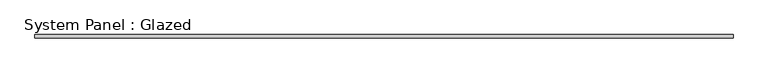
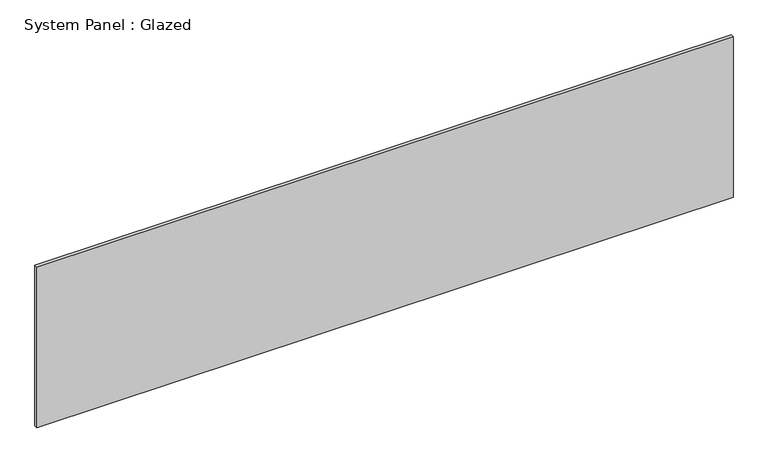
"""IFC4 building model written with IfcOpenShell, lengths in millimetres: plate geometry, System Panel : Glazed."""

from ifc_helpers import new_model, si_unit, origin, origin_with_axes, place, context, project, spatial, polyline, outline, extrude, source, transform, mapped, element, save


def system_panel_glazed_21a5631f(model_context):
    return source(origin(), model_context, "Body", "SweptSolid", [
        extrude(outline(polyline([(2501.9, 19.05), (-2501.9, 19.05), (-2501.9, 44.45), (2501.9, 44.45), (2501.9, 19.05)])), origin_with_axes(), (0.0, 0.0, 1.0), 1219.2),
    ])


if __name__ == "__main__":
    model = new_model("IFC4")
    model_context = context("Model", 3, world=origin())
    ifc_project = project(units=[si_unit("LENGTHUNIT", "METRE", prefix="MILLI")], contexts=[model_context])
    site = spatial("IfcSite", under=ifc_project)
    building = spatial("IfcBuilding", under=site)
    placement = place(None, origin())
    system_panel_glazed_shape = system_panel_glazed_21a5631f(model_context)
    element("IfcPlate", 1, ObjectType="System Panel : Glazed", at=placement, inside=building, context=model_context, shape_type="MappedRepresentation", body=[
        mapped(system_panel_glazed_shape, transform((0.0, 0.0, 0.0), x_axis=(1.0, 0.0, 0.0), y_axis=(0.0, 1.0, 0.0), z_axis=(0.0, 0.0, 1.0))),
    ])
    save(model, "model.ifc")

# Revit data of these elements
# Type "System Panel : Glazed"
#   Construction Type Id = "GSP4R"
#   Analytic Construction = "1/8 in Pilkington single glazing"
#   Visual Light Transmittance = 0.9
#   Solar Heat Gain Coefficient = 0.86
#   Heat Transfer Coefficient (U) = 1.18115 BTU/(h·ft²·°F)
# Element 1 (IfcPlate, "System Panel : Glazed")
#   Materials on its faces: "Glass"
# Materials
#   "Glass": class "Glass", colour RGB 0 128 192, transparency 0.75, Description = "Soda Lime Glass", Cost = 0
